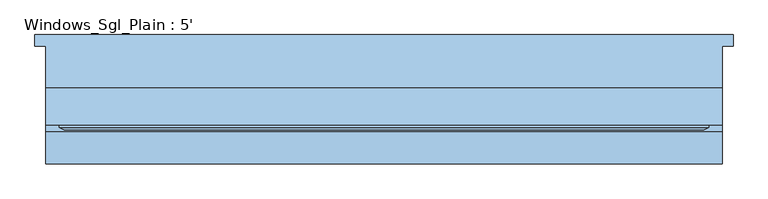
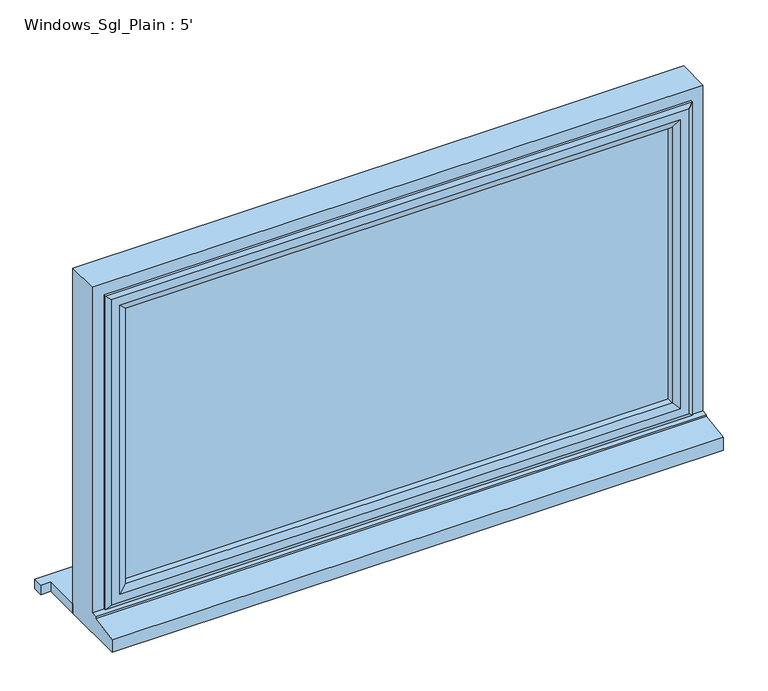
"""IFC4 building model written with IfcOpenShell, lengths in millimetres: window geometry, Windows_Sgl_Plain : 5'."""

from ifc_helpers import new_model, si_unit, frame, origin, place, context, project, spatial, polyline, outline, extrude, faceted_brep, source, transform, mapped, element, save


def windows_sgl_plain_5_c2f68037(model_context):
    return source(origin(), model_context, "Body", "SolidModel", [
        extrude(outline(polyline([(-787.0, 130.8434322), (787.0, 130.8434322), (787.0, 105.8434322), (762.0, 105.8434322), (762.0, 10.2434322), (-762.0, 10.2434322), (-762.0, 105.8434322), (-787.0, 105.8434322), (-787.0, 130.8434322)])), frame((0.0, 0.0, 1200.0), z_axis=(0.0, 0.0, 1.0), x_axis=(1.0, 0.0, 0.0)), (0.0, 0.0, 1.0), 25.0),
        faceted_brep([(-762.0, 10.2434322, 1200.0), (-762.0, 10.2434322, 2110.0), (762.0, 10.2434322, 2110.0), (762.0, 10.2434322, 1200.0), (-702.0, 10.2434322, 2050.0), (-702.0, 10.2434322, 1275.0), (702.0, 10.2434322, 1275.0), (702.0, 10.2434322, 2050.0), (-762.0, -160.2565678, 1200.0), (-762.0, -160.2565678, 1233.8088847), (-762.0, -87.7565678, 1244.7449676), (-762.0, -87.7565678, 1249.68767), (-762.0, -72.7565678, 1251.0), (-762.0, -72.7565678, 2110.0), (762.0, -72.7565678, 1251.0), (762.0, -72.7565678, 2110.0), (-722.0, -72.7565678, 2070.0), (722.0, -72.7565678, 2070.0), (722.0, -72.7565678, 1263.0), (-722.0, -72.7565678, 1263.0), (-722.0, -7.7565678, 1263.0), (-722.0, -7.7565678, 2070.0), (722.0, -7.7565678, 1263.0), (722.0, -7.7565678, 2070.0), (-702.0, -7.7565678, 2050.0), (702.0, -7.7565678, 2050.0), (702.0, -7.7565678, 1275.0), (-702.0, -7.7565678, 1275.0), (762.0, -87.7565678, 1249.68767), (762.0, -87.7565678, 1244.7449676), (762.0, -160.2565678, 1233.8088847), (762.0, -160.2565678, 1200.0)], [[[0, 1, 2, 3], [4, 5, 6, 7]], [[0, 8, 9, 10, 11, 12, 13, 1]], [[12, 14, 15, 13], [16, 17, 18, 19]], [[19, 20, 21, 16]], [[21, 20, 22, 23], [24, 25, 26, 27]], [[24, 27, 5, 4]], [[1, 13, 15, 2]], [[16, 21, 23, 17]], [[7, 25, 24, 4]], [[14, 28, 29, 30, 31, 3, 2, 15]], [[17, 23, 22, 18]], [[7, 6, 26, 25]], [[31, 8, 0, 3]], [[30, 9, 8, 31]], [[29, 10, 9, 30]], [[28, 11, 10, 29]], [[14, 12, 11, 28]], [[20, 19, 18, 22]], [[5, 27, 26, 6]]]),
        extrude(outline(polyline([(692.0, -36.7565678), (692.0, -60.7565678), (-692.0, -60.7565678), (-692.0, -36.7565678), (692.0, -36.7565678)])), frame((0.0, 0.0, 1293.0), z_axis=(0.0, 0.0, 1.0), x_axis=(1.0, 0.0, 0.0)), (0.0, 0.0, 1.0), 747.0),
        faceted_brep([(-732.0, -72.7565678, 2080.0), (-732.0, -72.7565678, 1253.0), (-732.0, -78.5300705, 1253.0), (-732.0, -78.5300705, 2080.0), (-722.0, -7.7565678, 2070.0), (-722.0, -7.7565678, 1263.0), (-722.0, -72.7565678, 1263.0), (-722.0, -72.7565678, 2070.0), (-682.0, -22.2494677, 2030.0), (-682.0, -22.2494677, 1303.0), (-692.1480377, -7.7565678, 1292.8519623), (-692.1480377, -7.7565678, 2040.1480377), (-682.0, -36.7565678, 2030.0), (-682.0, -36.7565678, 1303.0), (-692.0, -60.7565678, 2040.0), (-692.0, -60.7565678, 1293.0), (-692.0, -36.7565678, 1293.0), (-692.0, -36.7565678, 2040.0), (-682.0, -78.5300705, 2030.0), (-682.0, -78.5300705, 1303.0), (-682.0, -60.7565678, 1303.0), (-682.0, -60.7565678, 2030.0), (-699.4457548, -84.3035732, 2047.4457548), (-699.4457548, -84.3035732, 1285.5542452), (-721.2153903, -84.3035732, 1263.7846097), (-721.2153903, -84.3035732, 2069.2153903), (732.0, -72.7565678, 1253.0), (732.0, -78.5300705, 1253.0), (722.0, -7.7565678, 1263.0), (722.0, -72.7565678, 1263.0), (682.0, -22.2494677, 1303.0), (692.1480377, -7.7565678, 1292.8519623), (682.0, -36.7565678, 1303.0), (692.0, -60.7565678, 1293.0), (692.0, -36.7565678, 1293.0), (682.0, -78.5300705, 1303.0), (682.0, -60.7565678, 1303.0), (699.4457548, -84.3035732, 1285.5542452), (721.2153903, -84.3035732, 1263.7846097), (732.0, -72.7565678, 2080.0), (732.0, -78.5300705, 2080.0), (722.0, -7.7565678, 2070.0), (722.0, -72.7565678, 2070.0), (682.0, -22.2494677, 2030.0), (692.1480377, -7.7565678, 2040.1480377), (682.0, -36.7565678, 2030.0), (692.0, -60.7565678, 2040.0), (692.0, -36.7565678, 2040.0), (682.0, -78.5300705, 2030.0), (682.0, -60.7565678, 2030.0), (699.4457548, -84.3035732, 2047.4457548), (721.2153903, -84.3035732, 2069.2153903)], [[[0, 1, 2, 3]], [[4, 5, 6, 7]], [[8, 9, 10, 11]], [[12, 13, 9, 8]], [[14, 15, 16, 17]], [[18, 19, 20, 21]], [[22, 23, 19, 18]], [[3, 2, 24, 25]], [[1, 26, 27, 2]], [[5, 28, 29, 6]], [[9, 30, 31, 10]], [[13, 32, 30, 9]], [[15, 33, 34, 16]], [[19, 35, 36, 20]], [[23, 37, 35, 19]], [[2, 27, 38, 24]], [[26, 39, 40, 27]], [[28, 41, 42, 29]], [[30, 43, 44, 31]], [[32, 45, 43, 30]], [[33, 46, 47, 34]], [[35, 48, 49, 36]], [[37, 50, 48, 35]], [[27, 40, 51, 38]], [[39, 0, 3, 40]], [[1, 0, 39, 26], [7, 6, 29, 42]], [[41, 4, 7, 42]], [[5, 4, 41, 28], [11, 10, 31, 44]], [[43, 8, 11, 44]], [[45, 12, 8, 43]], [[17, 16, 34, 47], [13, 12, 45, 32]], [[46, 14, 17, 47]], [[15, 14, 46, 33], [21, 20, 36, 49]], [[48, 18, 21, 49]], [[50, 22, 18, 48]], [[25, 24, 38, 51], [23, 22, 50, 37]], [[40, 3, 25, 51]]]),
    ])


if __name__ == "__main__":
    model = new_model("IFC4")
    model_context = context("Model", 3, world=origin())
    ifc_project = project(units=[si_unit("LENGTHUNIT", "METRE", prefix="MILLI")], contexts=[model_context])
    site = spatial("IfcSite", under=ifc_project)
    building = spatial("IfcBuilding", under=site)
    placement = place(None, origin())
    windows_sgl_plain_5_shape = windows_sgl_plain_5_c2f68037(model_context)
    element("IfcWindow", 1, ObjectType="Windows_Sgl_Plain : 5'", at=placement, inside=building, context=model_context, shape_type="MappedRepresentation", body=[
        mapped(windows_sgl_plain_5_shape, transform((0.0, 0.0, 0.0), x_axis=(1.0, 0.0, 0.0), y_axis=(0.0, 1.0, 0.0), z_axis=(0.0, 0.0, 1.0))),
    ])
    save(model, "model.ifc")

# Revit data of these elements
# Type "Windows_Sgl_Plain : 5'"
#   Type Mark = "67"
#   Operation = "SinglePanel"
#   Construction Type Id = "SGL"
#   Manufacturer = "Revit"
#   Keynote = "L10"
#   Analytic Construction = "Large single-glazed windows"
#   Wrap Layers (Ext) from Ext = 0' - 4.03543"
#   Wrap Layers (Int) from Ext = 0' - 6.98819"
#   Window Board Projection = 0' - 0.98425"
#   Window Board Extension = 0' - 0.98425"
#   Visual Light Transmittance = 0.9
#   Solar Heat Gain Coefficient = 0.86
#   Rough Width = 5' - 0"
#   Rough Height = 2' - 11.82677"
#   Height = 2' - 11.82677"
#   Width = 5' - 0"
#   Heat Transfer Coefficient (U) = 5.5617 W/(m²·K)
#   Glazing Thickness = 0' - 0.94488"
#   FrameOffset - External = 0' - 1.9685"
#   Frame Depth = 0' - 2.55906"
#   Default Head Height = 6' - 11.07087"
#   Cill Depth = 0' - 3.44488"
#   Cavity Closer Width = 0' - 1.9685"
#   Cavity Closer Offset from Ext = 0' - 4.03543"
#   Cavity Closer Depth = 0' - 3.34646"
#   Vis - Cavity Closers = yes
#   Define Thermal Properties by = 1
#   Material Trim = Window Frame
#   Material Glass = Glass
#   Material Frame = Window Frame
#   Wall Closure = (empty or 0)
# Element 1 (IfcWindow, "Windows_Sgl_Plain : 5'")
#   Materials on its faces: "Window Frame", "Glass"
# Materials
#   "Window Frame": colour RGB 249 249 249, transparency 0, Keynote = "L10", Cost = 0
#   "Glass": class "Glass", colour RGB 0 128 192, transparency 0.9, Description = "Soda Lime Glass", Cost = 0
